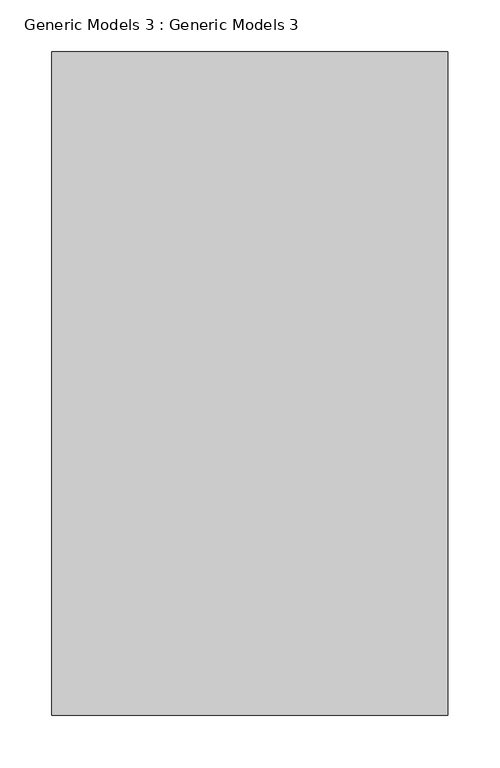
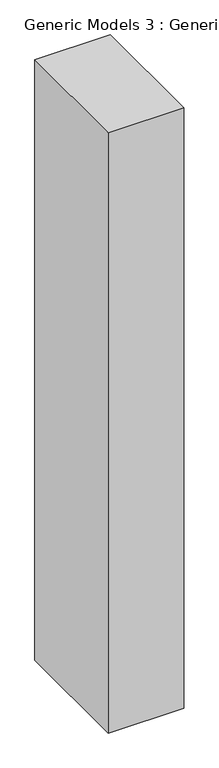
"""IFC4 building model written with IfcOpenShell, lengths in millimetres: proxy geometry, Generic Models 3 : Generic Models 3."""

from ifc_helpers import new_model, si_unit, frame, origin, place, context, project, spatial, polyline, outline, extrude, source, transform, mapped, element, save


def generic_models_3_generic_models_3_803ecd2f(model_context):
    return source(origin(), model_context, "Body", "SweptSolid", [
        extrude(outline(polyline([(-10125.8128458, 1851.619734), (-10125.8128458, 1212.7900127), (-10506.8128458, 1212.7900127), (-10506.8128458, 1851.619734), (-10125.8128458, 1851.619734)])), frame((0.0, 0.0, 3352.8), z_axis=(0.0, 0.0, 1.0), x_axis=(1.0, 0.0, 0.0)), (0.0, 0.0, 1.0), 3200.4),
    ])


if __name__ == "__main__":
    model = new_model("IFC4")
    model_context = context("Model", 3, world=origin())
    ifc_project = project(units=[si_unit("LENGTHUNIT", "METRE", prefix="MILLI")], contexts=[model_context])
    site = spatial("IfcSite", under=ifc_project)
    building = spatial("IfcBuilding", under=site)
    placement = place(None, origin())
    generic_models_3_generic_models_3_shape = generic_models_3_generic_models_3_803ecd2f(model_context)
    element("IfcBuildingElementProxy", 1, Name="Generic Models 3 : Generic Models 3", ObjectType="Generic Models 3 : Generic Models 3", at=placement, inside=building, context=model_context, shape_type="MappedRepresentation", body=[
        mapped(generic_models_3_generic_models_3_shape, transform((0.0, 0.0, 0.0), x_axis=(1.0, 0.0, 0.0), y_axis=(0.0, 1.0, 0.0), z_axis=(0.0, 0.0, 1.0))),
    ])
    save(model, "model.ifc")
